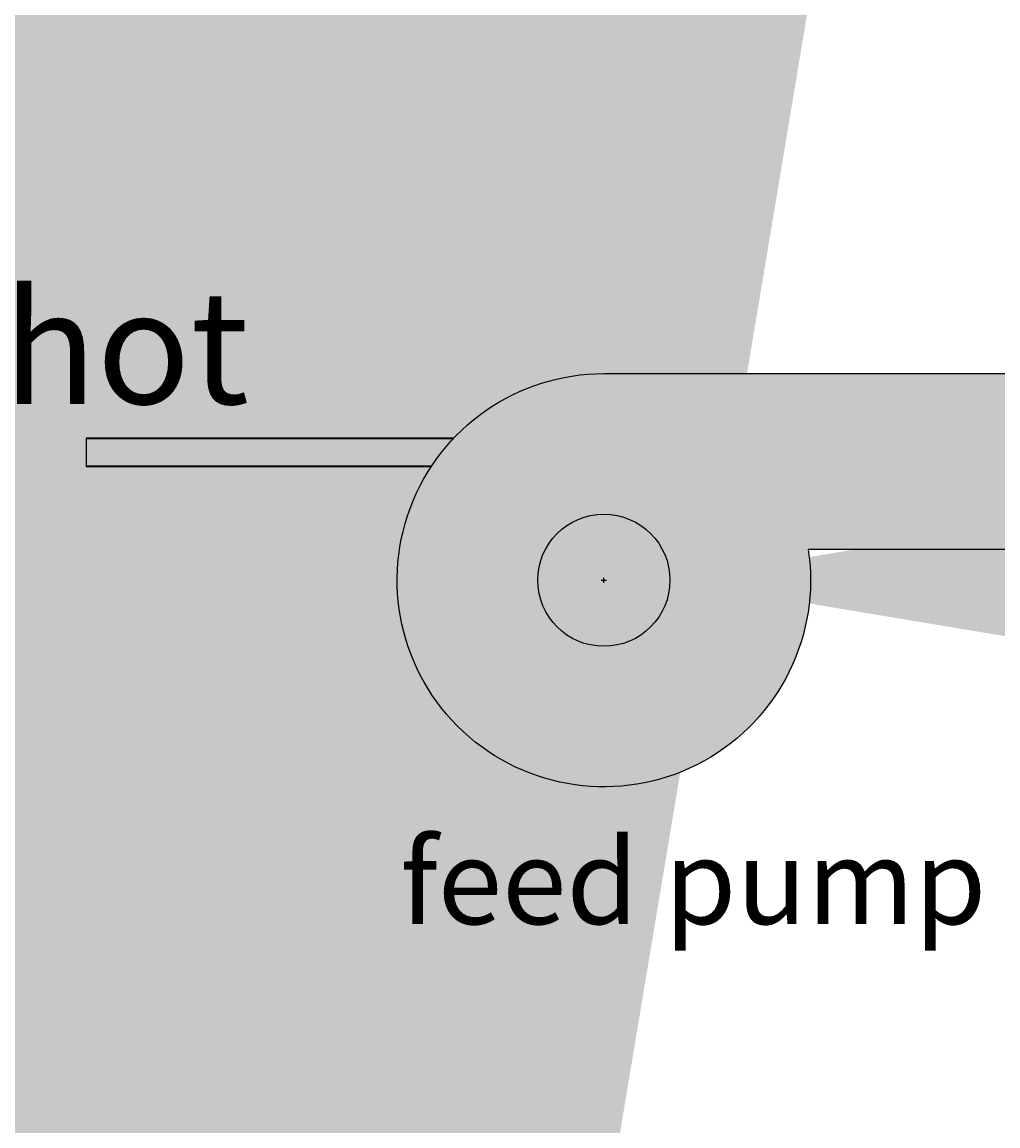
# Model space of a CAD drawing. Units: millimetres. Extents: x -22994 to 29398, y -19990 to 20176.
# Tile 23 of 135: x 37 to 71, y 99 to 138. Entities that reach past the tile are written whole.
import ezdxf

# ---------------------------------------------------------------- set-up
doc = ezdxf.new("R2010")
doc.units = ezdxf.units.MM
doc.header["$MEASUREMENT"] = 0
for name, color, linetype, lineweight in [('M-ANNO-TEXT', 7, 'Continuous', 25), ('M-DIMS', 2, 'Continuous', 18), ('M-EQPM', 7, 'Continuous', 25), ('M-EQPM-PATT', 7, 'Continuous', 18), ('M-PIPE', 7, 'Continuous', 35)]:
    doc.layers.add(name, color=color, linetype=linetype, lineweight=lineweight)
doc.styles.get("Standard").update_dxf_attribs({"font": 'arial.ttf'})
doc.dimstyles.get("Standard").update_dxf_attribs({"dimtxt": 0.18, "dimasz": 10000, "dimexe": 0.18, "dimexo": 0.0625, "dimgap": 0.09, "dimtad": 0, "dimtih": 1, "dimtoh": 1, "dimdec": 0, "dimzin": 0, "dimdsep": 46, "dimtxsty": 'Standard', "dimcen": 0.09, "dimadec": 0, "dimazin": 0, "dimtfac": 1, "dimtdec": 0, "dimtofl": 0, "dimtmove": 0, "dimatfit": 3, "dimfxl": 1, "dimtolj": 1, "dimtzin": 0, "dimlwd": 30, "dimarcsym": 0})

# ---------------------------------------------------------------- blocks, each defined once
blk = doc.blocks.new('*D2')
at = {"layer": 'Defpoints', "color": 0, "transparency": 16777216}
for p in [(6.677, 10.271), (290.852, 10.271), (290.852, -5.079)]:
    blk.add_point(p, dxfattribs=at)
at = {"layer": 'M-DIMS', "color": 0, "lineweight": -2, "transparency": 16777216}
for p, q in [((6.677, 10.209), (6.677, -5.259)), ((290.852, 10.209), (290.852, -5.259))]:
    blk.add_line(p, q, dxfattribs=at)
at = {"layer": 'M-DIMS', "color": 0, "lineweight": 30, "transparency": 16777216}
for p, q in [((-9993.323, -5.079), (-19993.323, -5.079)), ((10290.852, -5.079), (20290.852, -5.079))]:
    blk.add_line(p, q, dxfattribs=at)
at = {"layer": 'M-DIMS', "color": 0, "transparency": 16777216}
for points in [[(-9993.323, 1661.588), (-9993.323, -1671.745), (6.677, -5.079)], [(10290.852, 1661.588), (10290.852, -1671.745), (290.852, -5.079)]]:
    blk.add_solid(points, dxfattribs=at)
at = {"layer": 'M-DIMS', "color": 0, "transparency": 16777216, "insert": (148.765, -5.079), "char_height": 0.18, "attachment_point": 5}
blk.add_mtext('\\A1;284.2', dxfattribs=at)
blk = doc.blocks.new('*D3')
at = {"layer": 'Defpoints', "color": 0, "transparency": 16777216}
for p in [(110.265, 204.165), (110.265, 176.366), (95.833, 127.967)]:
    blk.add_point(p, dxfattribs=at)
at = {"layer": 'M-DIMS', "color": 0, "lineweight": -2, "transparency": 16777216}
for p, q in [((95.833, 128.03), (95.833, 204.345)), ((110.265, 176.429), (110.265, 204.345))]:
    blk.add_line(p, q, dxfattribs=at)
at = {"layer": 'M-DIMS', "color": 0, "lineweight": 30, "transparency": 16777216}
for p, q in [((-9904.167, 204.165), (-19904.167, 204.165)), ((10110.265, 204.165), (20110.265, 204.165))]:
    blk.add_line(p, q, dxfattribs=at)
at = {"layer": 'M-DIMS', "color": 0, "transparency": 16777216}
for points in [[(-9904.167, 1870.832), (-9904.167, -1462.501), (95.833, 204.165)], [(10110.265, 1870.832), (10110.265, -1462.501), (110.265, 204.165)]]:
    blk.add_solid(points, dxfattribs=at)
at = {"layer": 'M-DIMS', "color": 0, "transparency": 16777216, "insert": (103.049, 204.165), "char_height": 0.18, "attachment_point": 5}
blk.add_mtext('\\A1;14.432', dxfattribs=at)
blk = doc.blocks.new('*D4')
at = {"layer": 'Defpoints', "color": 0, "transparency": 16777216}
for p in [(116.265, 204.165), (110.265, 176.366), (116.265, 176.366)]:
    blk.add_point(p, dxfattribs=at)
at = {"layer": 'M-DIMS', "color": 0, "lineweight": -2, "transparency": 16777216}
for p, q in [((110.265, 176.429), (110.265, 204.345)), ((116.265, 176.429), (116.265, 204.345))]:
    blk.add_line(p, q, dxfattribs=at)
at = {"layer": 'M-DIMS', "color": 0, "lineweight": 30, "transparency": 16777216}
for p, q in [((-9889.735, 204.165), (-19889.735, 204.165)), ((10116.265, 204.165), (20116.265, 204.165))]:
    blk.add_line(p, q, dxfattribs=at)
at = {"layer": 'M-DIMS', "color": 0, "transparency": 16777216}
for points in [[(-9889.735, 1870.832), (-9889.735, -1462.501), (110.265, 204.165)], [(10116.265, 1870.832), (10116.265, -1462.501), (116.265, 204.165)]]:
    blk.add_solid(points, dxfattribs=at)
at = {"layer": 'M-DIMS', "color": 0, "transparency": 16777216, "insert": (113.265, 204.165), "char_height": 0.18, "attachment_point": 5}
blk.add_mtext('\\A1;6', dxfattribs=at)
blk = doc.blocks.new('*D5')
at = {"layer": 'Defpoints', "color": 0, "transparency": 16777216}
for p in [(181.265, 204.165), (116.265, 176.366), (181.265, 176.366)]:
    blk.add_point(p, dxfattribs=at)
at = {"layer": 'M-DIMS', "color": 0, "lineweight": -2, "transparency": 16777216}
for p, q in [((116.265, 176.429), (116.265, 204.345)), ((181.265, 176.429), (181.265, 204.345))]:
    blk.add_line(p, q, dxfattribs=at)
at = {"layer": 'M-DIMS', "color": 0, "lineweight": 30, "transparency": 16777216}
for p, q in [((-9883.735, 204.165), (-19883.735, 204.165)), ((10181.265, 204.165), (20181.265, 204.165))]:
    blk.add_line(p, q, dxfattribs=at)
at = {"layer": 'M-DIMS', "color": 0, "transparency": 16777216}
for points in [[(-9883.735, 1870.832), (-9883.735, -1462.501), (116.265, 204.165)], [(10181.265, 1870.832), (10181.265, -1462.501), (181.265, 204.165)]]:
    blk.add_solid(points, dxfattribs=at)
at = {"layer": 'M-DIMS', "color": 0, "transparency": 16777216, "insert": (148.765, 204.165), "char_height": 0.18, "attachment_point": 5}
blk.add_mtext('\\A1;65', dxfattribs=at)
blk = doc.blocks.new('*D6')
at = {"layer": 'Defpoints', "color": 0, "transparency": 16777216}
for p in [(187.265, 204.165), (181.265, 176.366), (187.265, 176.366)]:
    blk.add_point(p, dxfattribs=at)
at = {"layer": 'M-DIMS', "color": 0, "lineweight": -2, "transparency": 16777216}
for p, q in [((181.265, 176.429), (181.265, 204.345)), ((187.265, 176.429), (187.265, 204.345))]:
    blk.add_line(p, q, dxfattribs=at)
at = {"layer": 'M-DIMS', "color": 0, "lineweight": 30, "transparency": 16777216}
for p, q in [((-9818.735, 204.165), (-19818.735, 204.165)), ((10187.265, 204.165), (20187.265, 204.165))]:
    blk.add_line(p, q, dxfattribs=at)
at = {"layer": 'M-DIMS', "color": 0, "transparency": 16777216}
for points in [[(-9818.735, 1870.832), (-9818.735, -1462.501), (181.265, 204.165)], [(10187.265, 1870.832), (10187.265, -1462.501), (187.265, 204.165)]]:
    blk.add_solid(points, dxfattribs=at)
at = {"layer": 'M-DIMS', "color": 0, "transparency": 16777216, "insert": (184.265, 204.165), "char_height": 0.18, "attachment_point": 5}
blk.add_mtext('\\A1;6', dxfattribs=at)
blk = doc.blocks.new('*D7')
at = {"layer": 'Defpoints', "color": 0, "transparency": 16777216}
for p in [(201.697, 204.165), (187.265, 176.366), (201.697, 127.967)]:
    blk.add_point(p, dxfattribs=at)
at = {"layer": 'M-DIMS', "color": 0, "lineweight": -2, "transparency": 16777216}
for p, q in [((187.265, 176.429), (187.265, 204.345)), ((201.697, 128.03), (201.697, 204.345))]:
    blk.add_line(p, q, dxfattribs=at)
at = {"layer": 'M-DIMS', "color": 0, "lineweight": 30, "transparency": 16777216}
for p, q in [((-9812.735, 204.165), (-19812.735, 204.165)), ((10201.697, 204.165), (20201.697, 204.165))]:
    blk.add_line(p, q, dxfattribs=at)
at = {"layer": 'M-DIMS', "color": 0, "transparency": 16777216}
for points in [[(-9812.735, 1870.832), (-9812.735, -1462.501), (187.265, 204.165)], [(10201.697, 1870.832), (10201.697, -1462.501), (201.697, 204.165)]]:
    blk.add_solid(points, dxfattribs=at)
at = {"layer": 'M-DIMS', "color": 0, "transparency": 16777216, "insert": (194.481, 204.165), "char_height": 0.18, "attachment_point": 5}
blk.add_mtext('\\A1;14.432', dxfattribs=at)
blk = doc.blocks.new('*D8')
at = {"layer": 'Defpoints', "color": 0, "transparency": 16777216}
for p in [(227.648, 204.165), (227.648, 146.73), (201.697, 127.967)]:
    blk.add_point(p, dxfattribs=at)
at = {"layer": 'M-DIMS', "color": 0, "lineweight": -2, "transparency": 16777216}
for p, q in [((201.697, 128.03), (201.697, 204.345)), ((227.648, 146.792), (227.648, 204.345))]:
    blk.add_line(p, q, dxfattribs=at)
at = {"layer": 'M-DIMS', "color": 0, "lineweight": 30, "transparency": 16777216}
for p, q in [((-9798.303, 204.165), (-19798.303, 204.165)), ((10227.648, 204.165), (20227.648, 204.165))]:
    blk.add_line(p, q, dxfattribs=at)
at = {"layer": 'M-DIMS', "color": 0, "transparency": 16777216}
for points in [[(-9798.303, 1870.832), (-9798.303, -1462.501), (201.697, 204.165)], [(10227.648, 1870.832), (10227.648, -1462.501), (227.648, 204.165)]]:
    blk.add_solid(points, dxfattribs=at)
at = {"layer": 'M-DIMS', "color": 0, "transparency": 16777216, "insert": (214.673, 204.165), "char_height": 0.18, "attachment_point": 5}
blk.add_mtext('\\A1;25.95', dxfattribs=at)
blk = doc.blocks.new('*D9')
at = {"layer": 'Defpoints', "color": 0, "transparency": 16777216}
for p in [(187.265, 176.366), (306.202, 176.366), (290.852, 10.271)]:
    blk.add_point(p, dxfattribs=at)
at = {"layer": 'M-DIMS', "color": 0, "lineweight": 30, "transparency": 16777216}
for p, q in [((306.202, 10176.366), (306.202, 20176.366)), ((306.202, -9989.729), (306.202, -19989.729))]:
    blk.add_line(p, q, dxfattribs=at)
at = {"layer": 'M-DIMS', "color": 0, "lineweight": -2, "transparency": 16777216}
for p, q in [((187.327, 176.366), (306.382, 176.366)), ((290.915, 10.271), (306.382, 10.271))]:
    blk.add_line(p, q, dxfattribs=at)
at = {"layer": 'M-DIMS', "color": 0, "transparency": 16777216}
for points in [[(-1360.465, 10176.366), (1972.869, 10176.366), (306.202, 176.366)], [(-1360.465, -9989.729), (1972.869, -9989.729), (306.202, 10.271)]]:
    blk.add_solid(points, dxfattribs=at)
at = {"layer": 'M-DIMS', "color": 0, "transparency": 16777216, "insert": (306.202, 93.319), "char_height": 0.18, "attachment_point": 5}
blk.add_mtext('\\A1;166.1', dxfattribs=at)
blk = doc.blocks.new('*D10')
at = {"layer": 'Defpoints', "color": 0, "transparency": 16777216}
for p in [(125.65, 136.071), (133.346, 136.071), (133.346, -5.079)]:
    blk.add_point(p, dxfattribs=at)
at = {"layer": 'M-DIMS', "color": 0, "lineweight": -2, "transparency": 16777216}
for p, q in [((125.65, 136.009), (125.65, -5.259)), ((133.346, 136.009), (133.346, -5.259))]:
    blk.add_line(p, q, dxfattribs=at)
at = {"layer": 'M-DIMS', "color": 0, "lineweight": 30, "transparency": 16777216}
for p, q in [((-9874.35, -5.079), (-19874.35, -5.079)), ((10133.346, -5.079), (20133.346, -5.079))]:
    blk.add_line(p, q, dxfattribs=at)
at = {"layer": 'M-DIMS', "color": 0, "transparency": 16777216}
for points in [[(-9874.35, 1661.588), (-9874.35, -1671.745), (125.65, -5.079)], [(10133.346, 1661.588), (10133.346, -1671.745), (133.346, -5.079)]]:
    blk.add_solid(points, dxfattribs=at)
at = {"layer": 'M-DIMS', "color": 0, "transparency": 16777216, "insert": (129.498, -5.079), "char_height": 0.18, "attachment_point": 5}
blk.add_mtext('\\A1;7.696', dxfattribs=at)
blk = doc.blocks.new('*D11')
at = {"layer": 'Defpoints', "color": 0, "transparency": 16777216}
for p in [(133.346, 136.071), (135.65, 136.071), (135.65, -5.079)]:
    blk.add_point(p, dxfattribs=at)
at = {"layer": 'M-DIMS', "color": 0, "lineweight": -2, "transparency": 16777216}
for p, q in [((133.346, 136.009), (133.346, -5.259)), ((135.65, 136.009), (135.65, -5.259))]:
    blk.add_line(p, q, dxfattribs=at)
at = {"layer": 'M-DIMS', "color": 0, "lineweight": 30, "transparency": 16777216}
for p, q in [((-9866.654, -5.079), (-19866.654, -5.079)), ((10135.65, -5.079), (20135.65, -5.079))]:
    blk.add_line(p, q, dxfattribs=at)
at = {"layer": 'M-DIMS', "color": 0, "transparency": 16777216}
for points in [[(-9866.654, 1661.588), (-9866.654, -1671.745), (133.346, -5.079)], [(10135.65, 1661.588), (10135.65, -1671.745), (135.65, -5.079)]]:
    blk.add_solid(points, dxfattribs=at)
at = {"layer": 'M-DIMS', "color": 0, "transparency": 16777216, "insert": (134.498, -5.079), "char_height": 0.18, "attachment_point": 5}
blk.add_mtext('\\A1;2.304', dxfattribs=at)
blk = doc.blocks.new('*D12')
at = {"layer": 'Defpoints', "color": 0, "transparency": 16777216}
for p in [(135.65, 136.071), (145.65, 136.071), (145.65, -5.079)]:
    blk.add_point(p, dxfattribs=at)
at = {"layer": 'M-DIMS', "color": 0, "lineweight": -2, "transparency": 16777216}
for p, q in [((135.65, 136.009), (135.65, -5.259)), ((145.65, 136.009), (145.65, -5.259))]:
    blk.add_line(p, q, dxfattribs=at)
at = {"layer": 'M-DIMS', "color": 0, "lineweight": 30, "transparency": 16777216}
for p, q in [((-9864.35, -5.079), (-19864.35, -5.079)), ((10145.65, -5.079), (20145.65, -5.079))]:
    blk.add_line(p, q, dxfattribs=at)
at = {"layer": 'M-DIMS', "color": 0, "transparency": 16777216}
for points in [[(-9864.35, 1661.588), (-9864.35, -1671.745), (135.65, -5.079)], [(10145.65, 1661.588), (10145.65, -1671.745), (145.65, -5.079)]]:
    blk.add_solid(points, dxfattribs=at)
at = {"layer": 'M-DIMS', "color": 0, "transparency": 16777216, "insert": (140.65, -5.079), "char_height": 0.18, "attachment_point": 5}
blk.add_mtext('\\A1;10', dxfattribs=at)
blk = doc.blocks.new('*D13')
at = {"layer": 'Defpoints', "color": 0, "transparency": 16777216}
for p in [(145.65, 136.071), (155.65, 136.071), (155.65, -5.079)]:
    blk.add_point(p, dxfattribs=at)
at = {"layer": 'M-DIMS', "color": 0, "lineweight": -2, "transparency": 16777216}
for p, q in [((145.65, 136.009), (145.65, -5.259)), ((155.65, 136.009), (155.65, -5.259))]:
    blk.add_line(p, q, dxfattribs=at)
at = {"layer": 'M-DIMS', "color": 0, "lineweight": 30, "transparency": 16777216}
for p, q in [((-9854.35, -5.079), (-19854.35, -5.079)), ((10155.65, -5.079), (20155.65, -5.079))]:
    blk.add_line(p, q, dxfattribs=at)
at = {"layer": 'M-DIMS', "color": 0, "transparency": 16777216}
for points in [[(-9854.35, 1661.588), (-9854.35, -1671.745), (145.65, -5.079)], [(10155.65, 1661.588), (10155.65, -1671.745), (155.65, -5.079)]]:
    blk.add_solid(points, dxfattribs=at)
at = {"layer": 'M-DIMS', "color": 0, "transparency": 16777216, "insert": (150.65, -5.079), "char_height": 0.18, "attachment_point": 5}
blk.add_mtext('\\A1;10', dxfattribs=at)
blk = doc.blocks.new('*D14')
at = {"layer": 'Defpoints', "color": 0, "transparency": 16777216}
for p in [(155.65, 136.071), (165.65, 136.071), (165.65, -5.079)]:
    blk.add_point(p, dxfattribs=at)
at = {"layer": 'M-DIMS', "color": 0, "lineweight": -2, "transparency": 16777216}
for p, q in [((155.65, 136.009), (155.65, -5.259)), ((165.65, 136.009), (165.65, -5.259))]:
    blk.add_line(p, q, dxfattribs=at)
at = {"layer": 'M-DIMS', "color": 0, "lineweight": 30, "transparency": 16777216}
for p, q in [((-9844.35, -5.079), (-19844.35, -5.079)), ((10165.65, -5.079), (20165.65, -5.079))]:
    blk.add_line(p, q, dxfattribs=at)
at = {"layer": 'M-DIMS', "color": 0, "transparency": 16777216}
for points in [[(-9844.35, 1661.588), (-9844.35, -1671.745), (155.65, -5.079)], [(10165.65, 1661.588), (10165.65, -1671.745), (165.65, -5.079)]]:
    blk.add_solid(points, dxfattribs=at)
at = {"layer": 'M-DIMS', "color": 0, "transparency": 16777216, "insert": (160.65, -5.079), "char_height": 0.18, "attachment_point": 5}
blk.add_mtext('\\A1;10', dxfattribs=at)
blk = doc.blocks.new('*D15')
at = {"layer": 'Defpoints', "color": 0, "transparency": 16777216}
for p in [(173.346, 154.788), (173.346, 136.071), (306.202, 136.071)]:
    blk.add_point(p, dxfattribs=at)
at = {"layer": 'M-DIMS', "color": 0, "lineweight": 30, "transparency": 16777216}
for p, q in [((306.202, 10154.788), (306.202, 20154.788)), ((306.202, -9863.929), (306.202, -19863.929))]:
    blk.add_line(p, q, dxfattribs=at)
at = {"layer": 'M-DIMS', "color": 0, "lineweight": -2, "transparency": 16777216}
for p, q in [((173.408, 154.788), (306.382, 154.788)), ((173.408, 136.071), (306.382, 136.071))]:
    blk.add_line(p, q, dxfattribs=at)
at = {"layer": 'M-DIMS', "color": 0, "transparency": 16777216}
for points in [[(-1360.465, 10154.788), (1972.869, 10154.788), (306.202, 154.788)], [(-1360.465, -9863.929), (1972.869, -9863.929), (306.202, 136.071)]]:
    blk.add_solid(points, dxfattribs=at)
at = {"layer": 'M-DIMS', "color": 0, "transparency": 16777216, "insert": (306.202, 145.43), "char_height": 0.18, "attachment_point": 5}
blk.add_mtext('\\A1;18.717', dxfattribs=at)
blk = doc.blocks.new('*D16')
at = {"layer": 'Defpoints', "color": 0, "transparency": 16777216}
for p in [(120.17, 204.165), (110.466, 48.035), (120.17, 48.035)]:
    blk.add_point(p, dxfattribs=at)
at = {"layer": 'M-DIMS', "color": 0, "lineweight": -2, "transparency": 16777216}
for p, q in [((110.466, 48.097), (110.466, 204.345)), ((120.17, 48.097), (120.17, 204.345))]:
    blk.add_line(p, q, dxfattribs=at)
at = {"layer": 'M-DIMS', "color": 0, "lineweight": 30, "transparency": 16777216}
for p, q in [((-9889.534, 204.165), (-19889.534, 204.165)), ((10120.17, 204.165), (20120.17, 204.165))]:
    blk.add_line(p, q, dxfattribs=at)
at = {"layer": 'M-DIMS', "color": 0, "transparency": 16777216}
for points in [[(-9889.534, 1870.832), (-9889.534, -1462.501), (110.466, 204.165)], [(10120.17, 1870.832), (10120.17, -1462.501), (120.17, 204.165)]]:
    blk.add_solid(points, dxfattribs=at)
at = {"layer": 'M-DIMS', "color": 0, "transparency": 16777216, "insert": (115.318, 204.165), "char_height": 0.18, "attachment_point": 5}
blk.add_mtext('\\A1;9.704', dxfattribs=at)
blk = doc.blocks.new('*D17')
at = {"layer": 'Defpoints', "color": 0, "transparency": 16777216}
for p in [(126.17, 204.165), (120.17, 48.035), (126.17, 48.035)]:
    blk.add_point(p, dxfattribs=at)
at = {"layer": 'M-DIMS', "color": 0, "lineweight": -2, "transparency": 16777216}
for p, q in [((120.17, 48.097), (120.17, 204.345)), ((126.17, 48.097), (126.17, 204.345))]:
    blk.add_line(p, q, dxfattribs=at)
at = {"layer": 'M-DIMS', "color": 0, "lineweight": 30, "transparency": 16777216}
for p, q in [((-9879.83, 204.165), (-19879.83, 204.165)), ((10126.17, 204.165), (20126.17, 204.165))]:
    blk.add_line(p, q, dxfattribs=at)
at = {"layer": 'M-DIMS', "color": 0, "transparency": 16777216}
for points in [[(-9879.83, 1870.832), (-9879.83, -1462.501), (120.17, 204.165)], [(10126.17, 1870.832), (10126.17, -1462.501), (126.17, 204.165)]]:
    blk.add_solid(points, dxfattribs=at)
at = {"layer": 'M-DIMS', "color": 0, "transparency": 16777216, "insert": (123.17, 204.165), "char_height": 0.18, "attachment_point": 5}
blk.add_mtext('\\A1;6', dxfattribs=at)
blk = doc.blocks.new('*D18')
at = {"layer": 'Defpoints', "color": 0, "transparency": 16777216}
for p in [(132.17, 204.165), (126.17, 48.035), (132.17, 48.035)]:
    blk.add_point(p, dxfattribs=at)
at = {"layer": 'M-DIMS', "color": 0, "lineweight": -2, "transparency": 16777216}
for p, q in [((126.17, 48.097), (126.17, 204.345)), ((132.17, 48.097), (132.17, 204.345))]:
    blk.add_line(p, q, dxfattribs=at)
at = {"layer": 'M-DIMS', "color": 0, "lineweight": 30, "transparency": 16777216}
for p, q in [((-9873.83, 204.165), (-19873.83, 204.165)), ((10132.17, 204.165), (20132.17, 204.165))]:
    blk.add_line(p, q, dxfattribs=at)
at = {"layer": 'M-DIMS', "color": 0, "transparency": 16777216}
for points in [[(-9873.83, 1870.832), (-9873.83, -1462.501), (126.17, 204.165)], [(10132.17, 1870.832), (10132.17, -1462.501), (132.17, 204.165)]]:
    blk.add_solid(points, dxfattribs=at)
at = {"layer": 'M-DIMS', "color": 0, "transparency": 16777216, "insert": (129.17, 204.165), "char_height": 0.18, "attachment_point": 5}
blk.add_mtext('\\A1;6', dxfattribs=at)
blk = doc.blocks.new('*D19')
at = {"layer": 'Defpoints', "color": 0, "transparency": 16777216}
for p in [(138.17, 204.165), (132.17, 48.035), (138.17, 48.035)]:
    blk.add_point(p, dxfattribs=at)
at = {"layer": 'M-DIMS', "color": 0, "lineweight": -2, "transparency": 16777216}
for p, q in [((132.17, 48.097), (132.17, 204.345)), ((138.17, 48.097), (138.17, 204.345))]:
    blk.add_line(p, q, dxfattribs=at)
at = {"layer": 'M-DIMS', "color": 0, "lineweight": 30, "transparency": 16777216}
for p, q in [((-9867.83, 204.165), (-19867.83, 204.165)), ((10138.17, 204.165), (20138.17, 204.165))]:
    blk.add_line(p, q, dxfattribs=at)
at = {"layer": 'M-DIMS', "color": 0, "transparency": 16777216}
for points in [[(-9867.83, 1870.832), (-9867.83, -1462.501), (132.17, 204.165)], [(10138.17, 1870.832), (10138.17, -1462.501), (138.17, 204.165)]]:
    blk.add_solid(points, dxfattribs=at)
at = {"layer": 'M-DIMS', "color": 0, "transparency": 16777216, "insert": (135.17, 204.165), "char_height": 0.18, "attachment_point": 5}
blk.add_mtext('\\A1;6', dxfattribs=at)
blk = doc.blocks.new('*D20')
at = {"layer": 'Defpoints', "color": 0, "transparency": 16777216}
for p in [(144.17, 204.165), (138.17, 48.035), (144.17, 48.035)]:
    blk.add_point(p, dxfattribs=at)
at = {"layer": 'M-DIMS', "color": 0, "lineweight": -2, "transparency": 16777216}
for p, q in [((138.17, 48.097), (138.17, 204.345)), ((144.17, 48.097), (144.17, 204.345))]:
    blk.add_line(p, q, dxfattribs=at)
at = {"layer": 'M-DIMS', "color": 0, "lineweight": 30, "transparency": 16777216}
for p, q in [((-9861.83, 204.165), (-19861.83, 204.165)), ((10144.17, 204.165), (20144.17, 204.165))]:
    blk.add_line(p, q, dxfattribs=at)
at = {"layer": 'M-DIMS', "color": 0, "transparency": 16777216}
for points in [[(-9861.83, 1870.832), (-9861.83, -1462.501), (138.17, 204.165)], [(10144.17, 1870.832), (10144.17, -1462.501), (144.17, 204.165)]]:
    blk.add_solid(points, dxfattribs=at)
at = {"layer": 'M-DIMS', "color": 0, "transparency": 16777216, "insert": (141.17, 204.165), "char_height": 0.18, "attachment_point": 5}
blk.add_mtext('\\A1;6', dxfattribs=at)
blk = doc.blocks.new('*D21')
at = {"layer": 'Defpoints', "color": 0, "transparency": 16777216}
for p in [(149.116, 204.165), (144.17, 48.035), (149.116, 48.035)]:
    blk.add_point(p, dxfattribs=at)
at = {"layer": 'M-DIMS', "color": 0, "lineweight": -2, "transparency": 16777216}
for p, q in [((144.17, 48.097), (144.17, 204.345)), ((149.116, 48.097), (149.116, 204.345))]:
    blk.add_line(p, q, dxfattribs=at)
at = {"layer": 'M-DIMS', "color": 0, "lineweight": 30, "transparency": 16777216}
for p, q in [((-9855.83, 204.165), (-19855.83, 204.165)), ((10149.116, 204.165), (20149.116, 204.165))]:
    blk.add_line(p, q, dxfattribs=at)
at = {"layer": 'M-DIMS', "color": 0, "transparency": 16777216}
for points in [[(-9855.83, 1870.832), (-9855.83, -1462.501), (144.17, 204.165)], [(10149.116, 1870.832), (10149.116, -1462.501), (149.116, 204.165)]]:
    blk.add_solid(points, dxfattribs=at)
at = {"layer": 'M-DIMS', "color": 0, "transparency": 16777216, "insert": (146.643, 204.165), "char_height": 0.18, "attachment_point": 5}
blk.add_mtext('\\A1;4.945', dxfattribs=at)
blk = doc.blocks.new('*D22')
at = {"layer": 'Defpoints', "color": 0, "transparency": 16777216}
for p in [(149.116, 30.99), (155.116, 30.99), (155.116, -5.079)]:
    blk.add_point(p, dxfattribs=at)
at = {"layer": 'M-DIMS', "color": 0, "lineweight": -2, "transparency": 16777216}
for p, q in [((149.116, 30.927), (149.116, -5.259)), ((155.116, 30.927), (155.116, -5.259))]:
    blk.add_line(p, q, dxfattribs=at)
at = {"layer": 'M-DIMS', "color": 0, "lineweight": 30, "transparency": 16777216}
for p, q in [((-9850.884, -5.079), (-19850.884, -5.079)), ((10155.116, -5.079), (20155.116, -5.079))]:
    blk.add_line(p, q, dxfattribs=at)
at = {"layer": 'M-DIMS', "color": 0, "transparency": 16777216}
for points in [[(-9850.884, 1661.588), (-9850.884, -1671.745), (149.116, -5.079)], [(10155.116, 1661.588), (10155.116, -1671.745), (155.116, -5.079)]]:
    blk.add_solid(points, dxfattribs=at)
at = {"layer": 'M-DIMS', "color": 0, "transparency": 16777216, "insert": (152.116, -5.079), "char_height": 0.18, "attachment_point": 5}
blk.add_mtext('\\A1;6', dxfattribs=at)
blk = doc.blocks.new('*D23')
at = {"layer": 'Defpoints', "color": 0, "transparency": 16777216}
for p in [(155.116, 30.99), (161.116, 30.99), (161.116, -5.079)]:
    blk.add_point(p, dxfattribs=at)
at = {"layer": 'M-DIMS', "color": 0, "lineweight": -2, "transparency": 16777216}
for p, q in [((155.116, 30.927), (155.116, -5.259)), ((161.116, 30.927), (161.116, -5.259))]:
    blk.add_line(p, q, dxfattribs=at)
at = {"layer": 'M-DIMS', "color": 0, "lineweight": 30, "transparency": 16777216}
for p, q in [((-9844.884, -5.079), (-19844.884, -5.079)), ((10161.116, -5.079), (20161.116, -5.079))]:
    blk.add_line(p, q, dxfattribs=at)
at = {"layer": 'M-DIMS', "color": 0, "transparency": 16777216}
for points in [[(-9844.884, 1661.588), (-9844.884, -1671.745), (155.116, -5.079)], [(10161.116, 1661.588), (10161.116, -1671.745), (161.116, -5.079)]]:
    blk.add_solid(points, dxfattribs=at)
at = {"layer": 'M-DIMS', "color": 0, "transparency": 16777216, "insert": (158.116, -5.079), "char_height": 0.18, "attachment_point": 5}
blk.add_mtext('\\A1;6', dxfattribs=at)
blk = doc.blocks.new('*D24')
at = {"layer": 'Defpoints', "color": 0, "transparency": 16777216}
for p in [(161.116, 30.99), (166.439, 30.99), (166.439, -5.079)]:
    blk.add_point(p, dxfattribs=at)
at = {"layer": 'M-DIMS', "color": 0, "lineweight": -2, "transparency": 16777216}
for p, q in [((161.116, 30.927), (161.116, -5.259)), ((166.439, 30.927), (166.439, -5.259))]:
    blk.add_line(p, q, dxfattribs=at)
at = {"layer": 'M-DIMS', "color": 0, "lineweight": 30, "transparency": 16777216}
for p, q in [((-9838.884, -5.079), (-19838.884, -5.079)), ((10166.439, -5.079), (20166.439, -5.079))]:
    blk.add_line(p, q, dxfattribs=at)
at = {"layer": 'M-DIMS', "color": 0, "transparency": 16777216}
for points in [[(-9838.884, 1661.588), (-9838.884, -1671.745), (161.116, -5.079)], [(10166.439, 1661.588), (10166.439, -1671.745), (166.439, -5.079)]]:
    blk.add_solid(points, dxfattribs=at)
at = {"layer": 'M-DIMS', "color": 0, "transparency": 16777216, "insert": (163.777, -5.079), "char_height": 0.18, "attachment_point": 5}
blk.add_mtext('\\A1;5.323', dxfattribs=at)
blk = doc.blocks.new('*D25')
at = {"layer": 'Defpoints', "color": 0, "transparency": 16777216}
for p in [(166.439, 30.99), (172.439, 30.99), (172.439, -5.079)]:
    blk.add_point(p, dxfattribs=at)
at = {"layer": 'M-DIMS', "color": 0, "lineweight": -2, "transparency": 16777216}
for p, q in [((166.439, 30.927), (166.439, -5.259)), ((172.439, 30.927), (172.439, -5.259))]:
    blk.add_line(p, q, dxfattribs=at)
at = {"layer": 'M-DIMS', "color": 0, "lineweight": 30, "transparency": 16777216}
for p, q in [((-9833.561, -5.079), (-19833.561, -5.079)), ((10172.439, -5.079), (20172.439, -5.079))]:
    blk.add_line(p, q, dxfattribs=at)
at = {"layer": 'M-DIMS', "color": 0, "transparency": 16777216}
for points in [[(-9833.561, 1661.588), (-9833.561, -1671.745), (166.439, -5.079)], [(10172.439, 1661.588), (10172.439, -1671.745), (172.439, -5.079)]]:
    blk.add_solid(points, dxfattribs=at)
at = {"layer": 'M-DIMS', "color": 0, "transparency": 16777216, "insert": (169.439, -5.079), "char_height": 0.18, "attachment_point": 5}
blk.add_mtext('\\A1;6', dxfattribs=at)
blk = doc.blocks.new('*D26')
at = {"layer": 'Defpoints', "color": 0, "transparency": 16777216}
for p in [(172.439, 30.99), (178.439, 30.99), (178.439, -5.079)]:
    blk.add_point(p, dxfattribs=at)
at = {"layer": 'M-DIMS', "color": 0, "lineweight": -2, "transparency": 16777216}
for p, q in [((172.439, 30.927), (172.439, -5.259)), ((178.439, 30.927), (178.439, -5.259))]:
    blk.add_line(p, q, dxfattribs=at)
at = {"layer": 'M-DIMS', "color": 0, "lineweight": 30, "transparency": 16777216}
for p, q in [((-9827.561, -5.079), (-19827.561, -5.079)), ((10178.439, -5.079), (20178.439, -5.079))]:
    blk.add_line(p, q, dxfattribs=at)
at = {"layer": 'M-DIMS', "color": 0, "transparency": 16777216}
for points in [[(-9827.561, 1661.588), (-9827.561, -1671.745), (172.439, -5.079)], [(10178.439, 1661.588), (10178.439, -1671.745), (178.439, -5.079)]]:
    blk.add_solid(points, dxfattribs=at)
at = {"layer": 'M-DIMS', "color": 0, "transparency": 16777216, "insert": (175.439, -5.079), "char_height": 0.18, "attachment_point": 5}
blk.add_mtext('\\A1;6', dxfattribs=at)
blk = doc.blocks.new('*D27')
at = {"layer": 'Defpoints', "color": 0, "transparency": 16777216}
for p in [(178.439, 30.99), (188.117, 30.99), (188.117, -5.079)]:
    blk.add_point(p, dxfattribs=at)
at = {"layer": 'M-DIMS', "color": 0, "lineweight": -2, "transparency": 16777216}
for p, q in [((178.439, 30.927), (178.439, -5.259)), ((188.117, 30.927), (188.117, -5.259))]:
    blk.add_line(p, q, dxfattribs=at)
at = {"layer": 'M-DIMS', "color": 0, "lineweight": 30, "transparency": 16777216}
for p, q in [((-9821.561, -5.079), (-19821.561, -5.079)), ((10188.117, -5.079), (20188.117, -5.079))]:
    blk.add_line(p, q, dxfattribs=at)
at = {"layer": 'M-DIMS', "color": 0, "transparency": 16777216}
for points in [[(-9821.561, 1661.588), (-9821.561, -1671.745), (178.439, -5.079)], [(10188.117, 1661.588), (10188.117, -1671.745), (188.117, -5.079)]]:
    blk.add_solid(points, dxfattribs=at)
at = {"layer": 'M-DIMS', "color": 0, "transparency": 16777216, "insert": (183.278, -5.079), "char_height": 0.18, "attachment_point": 5}
blk.add_mtext('\\A1;9.679', dxfattribs=at)
blk = doc.blocks.new('*D28')
at = {"layer": 'Defpoints', "color": 0, "transparency": 16777216}
for p in [(188.117, 48.035), (306.202, 48.035), (188.117, 30.99)]:
    blk.add_point(p, dxfattribs=at)
at = {"layer": 'M-DIMS', "color": 0, "lineweight": 30, "transparency": 16777216}
for p, q in [((306.202, 10048.035), (306.202, 20048.035)), ((306.202, -9969.01), (306.202, -19969.01))]:
    blk.add_line(p, q, dxfattribs=at)
at = {"layer": 'M-DIMS', "color": 0, "lineweight": -2, "transparency": 16777216}
for p, q in [((188.18, 48.035), (306.382, 48.035)), ((188.18, 30.99), (306.382, 30.99))]:
    blk.add_line(p, q, dxfattribs=at)
at = {"layer": 'M-DIMS', "color": 0, "transparency": 16777216}
for points in [[(-1360.465, 10048.035), (1972.869, 10048.035), (306.202, 48.035)], [(-1360.465, -9969.01), (1972.869, -9969.01), (306.202, 30.99)]]:
    blk.add_solid(points, dxfattribs=at)
at = {"layer": 'M-DIMS', "color": 0, "transparency": 16777216, "insert": (306.202, 39.512), "char_height": 0.18, "attachment_point": 5}
blk.add_mtext('\\A1;17.045', dxfattribs=at)
blk = doc.blocks.new('*D29')
at = {"layer": 'Defpoints', "color": 0, "transparency": 16777216}
for p in [(36.801, 80.045), (64.03, 80.045)]:
    blk.add_point(p, dxfattribs=at)
at = {"layer": 'M-DIMS', "color": 0, "lineweight": -2, "transparency": 16777216}
for p, q in [((50.325, 80.045), (50.505, 80.045)), ((50.415, 79.955), (50.415, 80.135))]:
    blk.add_line(p, q, dxfattribs=at)
at = {"layer": 'M-DIMS', "color": 0, "lineweight": 30, "transparency": 16777216}
blk.add_line((20064.03, 80.03), (10064.03, 80.038), dxfattribs=at)
at = {"layer": 'M-DIMS', "color": 0, "transparency": 16777216}
blk.add_solid([(10064.031, 1746.704), (10064.028, -1586.629), (64.03, 80.045)], dxfattribs=at)
at = {"layer": 'M-DIMS', "color": 0, "transparency": 16777216, "insert": (20064.521, 80.03), "char_height": 0.18, "attachment_point": 5}
blk.add_mtext('\\A1;∅27.23', dxfattribs=at)
blk = doc.blocks.new('*D32')
at = {"layer": 'Defpoints', "color": 0, "transparency": 16777216}
for p in [(57.164, 118.614), (52.413, 113.093)]:
    blk.add_point(p, dxfattribs=at)
at = {"layer": 'M-DIMS', "color": 0, "lineweight": -2, "transparency": 16777216}
for p, q in [((57.164, 118.524), (57.164, 118.704)), ((57.074, 118.614), (57.254, 118.614))]:
    blk.add_line(p, q, dxfattribs=at)
at = {"layer": 'M-DIMS', "color": 0, "lineweight": 30, "transparency": 16777216}
for p, q in [((-12992.534, -15047.031), (-6470.06, -7466.969)), ((-22992.534, -15047.031), (-12992.534, -15047.031))]:
    blk.add_line(p, q, dxfattribs=at)
at = {"layer": 'M-DIMS', "color": 0, "transparency": 16777216}
blk.add_solid([(-7733.404, -6379.89), (-5206.717, -8554.048), (52.413, 113.093)], dxfattribs=at)
at = {"layer": 'M-DIMS', "color": 0, "transparency": 16777216, "insert": (-22993.208, -15047.031), "char_height": 0.18, "attachment_point": 5}
blk.add_mtext('\\A1;2X R7.284', dxfattribs=at)
blk = doc.blocks.new('*D36')
at = {"layer": 'Defpoints', "color": 0, "transparency": 16777216}
for p in [(46.39, 31.303), (46.387, 26.593)]:
    blk.add_point(p, dxfattribs=at)
at = {"layer": 'M-DIMS', "color": 0, "lineweight": 30, "transparency": 16777216}
for p, q in [((57.15, 20031.301), (51.77, 10031.302)), ((10057.15, 20031.301), (57.15, 20031.301))]:
    blk.add_line(p, q, dxfattribs=at)
at = {"layer": 'M-DIMS', "color": 0, "lineweight": -2, "transparency": 16777216}
for p, q in [((46.299, 28.948), (46.479, 28.948)), ((46.389, 28.858), (46.389, 29.038))]:
    blk.add_line(p, q, dxfattribs=at)
at = {"layer": 'M-DIMS', "color": 0, "transparency": 16777216}
blk.add_solid([(-1614.896, 10032.199), (1718.436, 10030.405), (46.39, 31.303)], dxfattribs=at)
at = {"layer": 'M-DIMS', "color": 0, "transparency": 16777216, "insert": (10057.554, 20031.301), "char_height": 0.18, "attachment_point": 5}
blk.add_mtext('\\A1;∅4.71', dxfattribs=at)
blk = doc.blocks.new('*D37')
at = {"layer": 'Defpoints', "color": 0, "transparency": 16777216}
for p in [(54.834, 118.615), (59.494, 118.614)]:
    blk.add_point(p, dxfattribs=at)
at = {"layer": 'M-DIMS', "color": 0, "lineweight": -2, "transparency": 16777216}
for p, q in [((57.164, 118.524), (57.164, 118.704)), ((57.074, 118.614), (57.254, 118.614))]:
    blk.add_line(p, q, dxfattribs=at)
at = {"layer": 'M-DIMS', "color": 0, "lineweight": 30, "transparency": 16777216}
blk.add_line((20059.493, 116.253), (10059.494, 117.434), dxfattribs=at)
at = {"layer": 'M-DIMS', "color": 0, "transparency": 16777216}
blk.add_solid([(10059.69, 1784.1), (10059.297, -1549.233), (59.494, 118.614)], dxfattribs=at)
at = {"layer": 'M-DIMS', "color": 0, "transparency": 16777216, "insert": (20059.985, 116.253), "char_height": 0.18, "attachment_point": 5}
blk.add_mtext('\\A1;∅4.659', dxfattribs=at)

msp = doc.modelspace()

# ---------------------------------------------------------------- hatches: boundary and pattern name
at = {"layer": 'M-EQPM-PATT'}
h = msp.add_hatch(color=256, dxfattribs=at)
h.set_gradient(color1=(242, 103, 34), color2=(242, 103, 34), tint=1, name='CYLINDER')
h.paths.add_polyline_path([(53.5912, 30.0354), (64.8905, 30.0354), (64.8905, 36.2325), (46.3887, 36.2325, 2.6954641)])
h.paths.add_polyline_path([(44.0337, 28.9485, -1), (48.7438, 28.9485, -1)], flags=16)
h.paths.add_polyline_path([(75.6657, 119.7012), (75.6657, 125.8983), (57.1639, 125.8983, 2.6954641), (64.3664, 119.7012)])
h.paths.add_polyline_path([(59.4936, 118.6143, -1), (54.8343, 118.6143, -1)], flags=16)
h = msp.add_hatch(color=256, dxfattribs=at)
h.set_gradient(color1=(34, 52, 110), color2=(41, 49, 137), tint=1, name='CYLINDER')
h.paths.add_polyline_path([(101.8327, 123.6277), (101.8327, 122.6277), (176.8123, 122.6277, -0.4142136), (178.3123, 121.1277), (178.3123, 119.1277, -0.4142136), (176.8123, 117.6277), (129.8123, 117.6277, 0.4142136), (128.3123, 116.1277), (128.3123, 114.1277, 0.4142136), (129.8123, 112.6277), (176.8123, 112.6277, -0.4142136), (178.3123, 111.1277), (178.3123, 109.1277, -0.4142136), (176.8123, 107.6277), (129.8123, 107.6277, 0.4142136), (128.3123, 106.1277), (128.3123, 104.1277, 0.4142136), (129.8123, 102.6277), (176.8123, 102.6277, -0.4142136), (178.3123, 101.1277), (178.3123, 99.1277, -0.4142136), (176.8123, 97.6277), (101.8327, 97.6277), (101.8327, 96.6277), (176.8123, 96.6277, 0.4142136), (179.3123, 99.1277), (179.3123, 101.1277, 0.4142136), (176.8123, 103.6277), (129.8123, 103.6277, -0.4142136), (129.3123, 104.1277), (129.3123, 106.1277, -0.4142136), (129.8123, 106.6277), (176.8123, 106.6277, 0.4142136), (179.3123, 109.1277), (179.3123, 111.1277, 0.4142136), (176.8123, 113.6277), (129.8123, 113.6277, -0.4142136), (129.3123, 114.1277), (129.3123, 116.1277, -0.4142136), (129.8123, 116.6277), (176.8123, 116.6277, 0.4142136), (179.3123, 119.1277), (179.3123, 121.1277, 0.4142136), (176.8123, 123.6277)])
h.paths.add_polyline_path([(75.6657, 123.6277), (75.6657, 122.6277), (95.8327, 122.6277), (95.8327, 123.6277)])
h.paths.add_polyline_path([(51.0853, 122.6277, -0.0439182), (51.8797, 123.6277), (38.9157, 123.6277), (38.9157, 122.6277)])
h.paths.add_polyline_path([(95.8327, 96.6277), (95.8327, 97.6277), (22.2694, 97.6277, 0.4142136), (20.7694, 96.1277), (20.7694, 89.8712, 0.4142136), (22.2694, 88.3712), (39.6435, 88.3712, -0.024152), (40.4967, 89.3712), (23.2694, 89.3712, -0.4142136), (21.7694, 90.8712), (21.7694, 95.1277, -0.4142136), (23.2694, 96.6277)])
h.paths.add_polyline_path([(137.7248, 106.4435), (168.6853, 106.4435), (168.6853, 114.6864), (137.7248, 114.6864)], flags=25)

# ---------------------------------------------------------------- linework, layer by layer
at = {"layer": 'M-EQPM'}
msp.add_line((38.9157, 123.6277), (38.9157, 122.6277), dxfattribs=at)
msp.add_lwpolyline([(57.1639, 125.8983), (75.6657, 125.8983), (75.6657, 119.7012), (64.3664, 119.7012, -2.6954641)], format="xyb", close=True, dxfattribs=at)
msp.add_circle((57.1639, 118.6143), 2.3296, dxfattribs=at)
at = {"layer": 'M-PIPE'}
msp.add_line((51.0853, 122.6277), (38.9157, 122.6277), dxfattribs=at)
msp.add_lwpolyline([(38.9157, 123.6277), (51.8797, 123.6277)], dxfattribs=at)

# ---------------------------------------------------------------- texts
at = {"layer": 'M-ANNO-TEXT', "attachment_point": 1}
for s, width, insert, char_height in [('water from hot \\Pwell', 57.451589, (6.6341, 128.828), 4), ('feed pump', 37.883315, (49.9786, 109.4904), 3)]:
    msp.add_mtext_dynamic_manual_height_columns(s, width=width, gutter_width=1, heights=[0], dxfattribs=dict(at, insert=insert, char_height=char_height))

# ---------------------------------------------------------------- dimensions: what is measured, and where the dimension line sits
at = {"layer": 'M-DIMS'}
for base, p1, p2, override, picture, middle in [((306.202, 176.3662), (290.852, 10.2713), (187.2647, 176.3662), {"dimdec": 1, "dimlfac": 1, "dimrnd": 0, "dimzin": 0, "dimdsep": 46, "dimlunit": 2}, '*D9', (306.202, 93.3187)), ((306.202, 136.0713), (173.3459, 154.788), (173.3459, 136.0713), {"dimdec": 3, "dimlfac": 1, "dimrnd": 0, "dimzin": 0, "dimdsep": 46, "dimlunit": 2}, '*D15', (306.202, 145.4297)), ((306.202, 48.0349), (188.1175, 30.9895), (188.1175, 48.0349), {"dimdec": 3, "dimlfac": 1, "dimrnd": 0, "dimzin": 0, "dimdsep": 46, "dimlunit": 2}, '*D28', (306.202, 39.5122))]:
    dim = msp.add_linear_dim(base=base, p1=p1, p2=p2, angle=90, dimstyle='Standard', override=override, dxfattribs=at)
    dim.commit()
    dim.dimension.update_dxf_attribs({"geometry": picture, "text_midpoint": middle})
dim = msp.add_diameter_dim_2p(p1=(46.3875, 26.5934), p2=(46.39, 31.3035), dimstyle='Standard', override={"dimdec": 2, "dimlfac": 1, "dimrnd": 0, "dimzin": 0, "dimdsep": 46, "dimlunit": 2}, dxfattribs=at)
dim.commit()
dim.dimension.update_dxf_attribs({"geometry": '*D36', "text_midpoint": (10057.5542, 20031.3006), "dimtype": 163})
for base, p1, p2, override, picture, middle in [((110.2647, 204.1654), (95.8327, 127.967), (110.2647, 176.3662), {"dimdec": 3, "dimlfac": 1, "dimrnd": 0, "dimzin": 0, "dimdsep": 46, "dimlunit": 2}, '*D3', (103.0487, 204.1654)), ((116.2647, 204.1654), (110.2647, 176.3662), (116.2647, 176.3662), {"dimdec": 0, "dimlfac": 1, "dimrnd": 0, "dimzin": 0, "dimdsep": 46, "dimlunit": 2}, '*D4', (113.2647, 204.1654)), ((120.1702, 204.1654), (110.4658, 48.0349), (120.1702, 48.0349), {"dimdec": 3, "dimlfac": 1, "dimrnd": 0, "dimzin": 0, "dimdsep": 46, "dimlunit": 2}, '*D16', (115.318, 204.1654)), ((181.2647, 204.1654), (116.2647, 176.3662), (181.2647, 176.3662), {"dimdec": 0, "dimlfac": 1, "dimrnd": 0, "dimzin": 0, "dimdsep": 46, "dimlunit": 2}, '*D5', (148.7647, 204.1654)), ((126.1702, 204.1654), (120.1702, 48.0349), (126.1702, 48.0349), {"dimdec": 0, "dimlfac": 1, "dimrnd": 0, "dimzin": 0, "dimdsep": 46, "dimlunit": 2}, '*D17', (123.1702, 204.1654)), ((132.1702, 204.1654), (126.1702, 48.0349), (132.1702, 48.0349), {"dimdec": 0, "dimlfac": 1, "dimrnd": 0, "dimzin": 0, "dimdsep": 46, "dimlunit": 2}, '*D18', (129.1702, 204.1654)), ((138.1702, 204.1654), (132.1702, 48.0349), (138.1702, 48.0349), {"dimdec": 0, "dimlfac": 1, "dimrnd": 0, "dimzin": 0, "dimdsep": 46, "dimlunit": 2}, '*D19', (135.1702, 204.1654)), ((144.1702, 204.1654), (138.1702, 48.0349), (144.1702, 48.0349), {"dimdec": 0, "dimlfac": 1, "dimrnd": 0, "dimzin": 0, "dimdsep": 46, "dimlunit": 2}, '*D20', (141.1702, 204.1654)), ((149.11567, 204.16539), (144.17023, 48.03494), (149.11567, 48.03494), {"dimdec": 3, "dimlfac": 1, "dimrnd": 0, "dimzin": 0, "dimdsep": 46, "dimlunit": 2}, '*D21', (146.64295, 204.16539)), ((187.2647, 204.1654), (181.2647, 176.3662), (187.2647, 176.3662), {"dimdec": 0, "dimlfac": 1, "dimrnd": 0, "dimzin": 0, "dimdsep": 46, "dimlunit": 2}, '*D6', (184.2647, 204.1654)), ((201.6967, 204.1654), (187.2647, 176.3662), (201.6967, 127.967), {"dimdec": 3, "dimlfac": 1, "dimrnd": 0, "dimzin": 0, "dimdsep": 46, "dimlunit": 2}, '*D7', (194.4807, 204.1654)), ((227.6485, 204.1654), (201.6967, 127.967), (227.6485, 146.7296), {"dimdec": 2, "dimlfac": 1, "dimrnd": 0, "dimzin": 0, "dimdsep": 46, "dimlunit": 2}, '*D8', (214.6726, 204.1654)), ((290.852, -5.0787), (6.6773, 10.2713), (290.852, 10.2713), {"dimdec": 1, "dimlfac": 1, "dimrnd": 0, "dimzin": 0, "dimdsep": 46, "dimlunit": 2}, '*D2', (148.7647, -5.0787)), ((133.3459, -5.0787), (125.6498, 136.0713), (133.3459, 136.0713), {"dimdec": 3, "dimlfac": 1, "dimrnd": 0, "dimzin": 0, "dimdsep": 46, "dimlunit": 2}, '*D10', (129.4978, -5.0787)), ((135.6498, -5.0787), (133.3459, 136.0713), (135.6498, 136.0713), {"dimdec": 3, "dimlfac": 1, "dimrnd": 0, "dimzin": 0, "dimdsep": 46, "dimlunit": 2}, '*D11', (134.4978, -5.0787)), ((145.6498, -5.0787), (135.6498, 136.0713), (145.6498, 136.0713), {"dimdec": 0, "dimlfac": 1, "dimrnd": 0, "dimzin": 0, "dimdsep": 46, "dimlunit": 2}, '*D12', (140.6498, -5.0787)), ((155.6498, -5.0787), (145.6498, 136.0713), (155.6498, 136.0713), {"dimdec": 0, "dimlfac": 1, "dimrnd": 0, "dimzin": 0, "dimdsep": 46, "dimlunit": 2}, '*D13', (150.6498, -5.0787)), ((155.1157, -5.0787), (149.1157, 30.9895), (155.1157, 30.9895), {"dimdec": 0, "dimlfac": 1, "dimrnd": 0, "dimzin": 0, "dimdsep": 46, "dimlunit": 2}, '*D22', (152.1157, -5.0787)), ((161.1157, -5.0787), (155.1157, 30.9895), (161.1157, 30.9895), {"dimdec": 0, "dimlfac": 1, "dimrnd": 0, "dimzin": 0, "dimdsep": 46, "dimlunit": 2}, '*D23', (158.1157, -5.0787)), ((165.6498, -5.0787), (155.6498, 136.0713), (165.6498, 136.0713), {"dimdec": 0, "dimlfac": 1, "dimrnd": 0, "dimzin": 0, "dimdsep": 46, "dimlunit": 2}, '*D14', (160.6498, -5.0787)), ((166.4387, -5.0787), (161.1157, 30.9895), (166.4387, 30.9895), {"dimdec": 3, "dimlfac": 1, "dimrnd": 0, "dimzin": 0, "dimdsep": 46, "dimlunit": 2}, '*D24', (163.7772, -5.0787)), ((172.4387, -5.0787), (166.4387, 30.9895), (172.4387, 30.9895), {"dimdec": 0, "dimlfac": 1, "dimrnd": 0, "dimzin": 0, "dimdsep": 46, "dimlunit": 2}, '*D25', (169.4387, -5.0787)), ((178.4387, -5.0787), (172.4387, 30.9895), (178.4387, 30.9895), {"dimdec": 0, "dimlfac": 1, "dimrnd": 0, "dimzin": 0, "dimdsep": 46, "dimlunit": 2}, '*D26', (175.4387, -5.0787)), ((188.1175, -5.0787), (178.4387, 30.9895), (188.1175, 30.9895), {"dimdec": 3, "dimlfac": 1, "dimrnd": 0, "dimzin": 0, "dimdsep": 46, "dimlunit": 2}, '*D27', (183.2781, -5.0787))]:
    dim = msp.add_linear_dim(base=base, p1=p1, p2=p2, dimstyle='Standard', override=override, dxfattribs=at)
    dim.commit()
    dim.dimension.update_dxf_attribs({"geometry": picture, "text_midpoint": middle})
for p1, p2, override, picture, middle in [((54.8343, 118.6145), (59.4936, 118.614), {"dimdec": 3, "dimlfac": 1, "dimrnd": 0, "dimzin": 0, "dimdsep": 46, "dimlunit": 2}, '*D37', (20059.4934, 116.2531)), ((36.8006, 80.045), (64.0296, 80.045), {"dimdec": 2, "dimlfac": 1, "dimrnd": 0, "dimzin": 0, "dimdsep": 46, "dimlunit": 2}, '*D29', (20064.0296, 80.0303))]:
    dim = msp.add_diameter_dim_2p(p1=p1, p2=p2, dimstyle='Standard', override=override, dxfattribs=at)
    dim.commit()
    dim.dimension.update_dxf_attribs({"geometry": picture, "text_midpoint": middle})
dim = msp.add_radius_dim(center=(57.1639, 118.6143), mpoint=(52.4129, 113.0929), text='2X <>', dimstyle='Standard', override={"dimdec": 3, "dimlfac": 1, "dimrnd": 0, "dimzin": 0, "dimdsep": 46, "dimlunit": 2}, dxfattribs=at)
dim.commit()
dim.dimension.update_dxf_attribs({"geometry": '*D32', "text_midpoint": (-22993.208, -15047.0314)})

doc.saveas('drawing.dxf')
